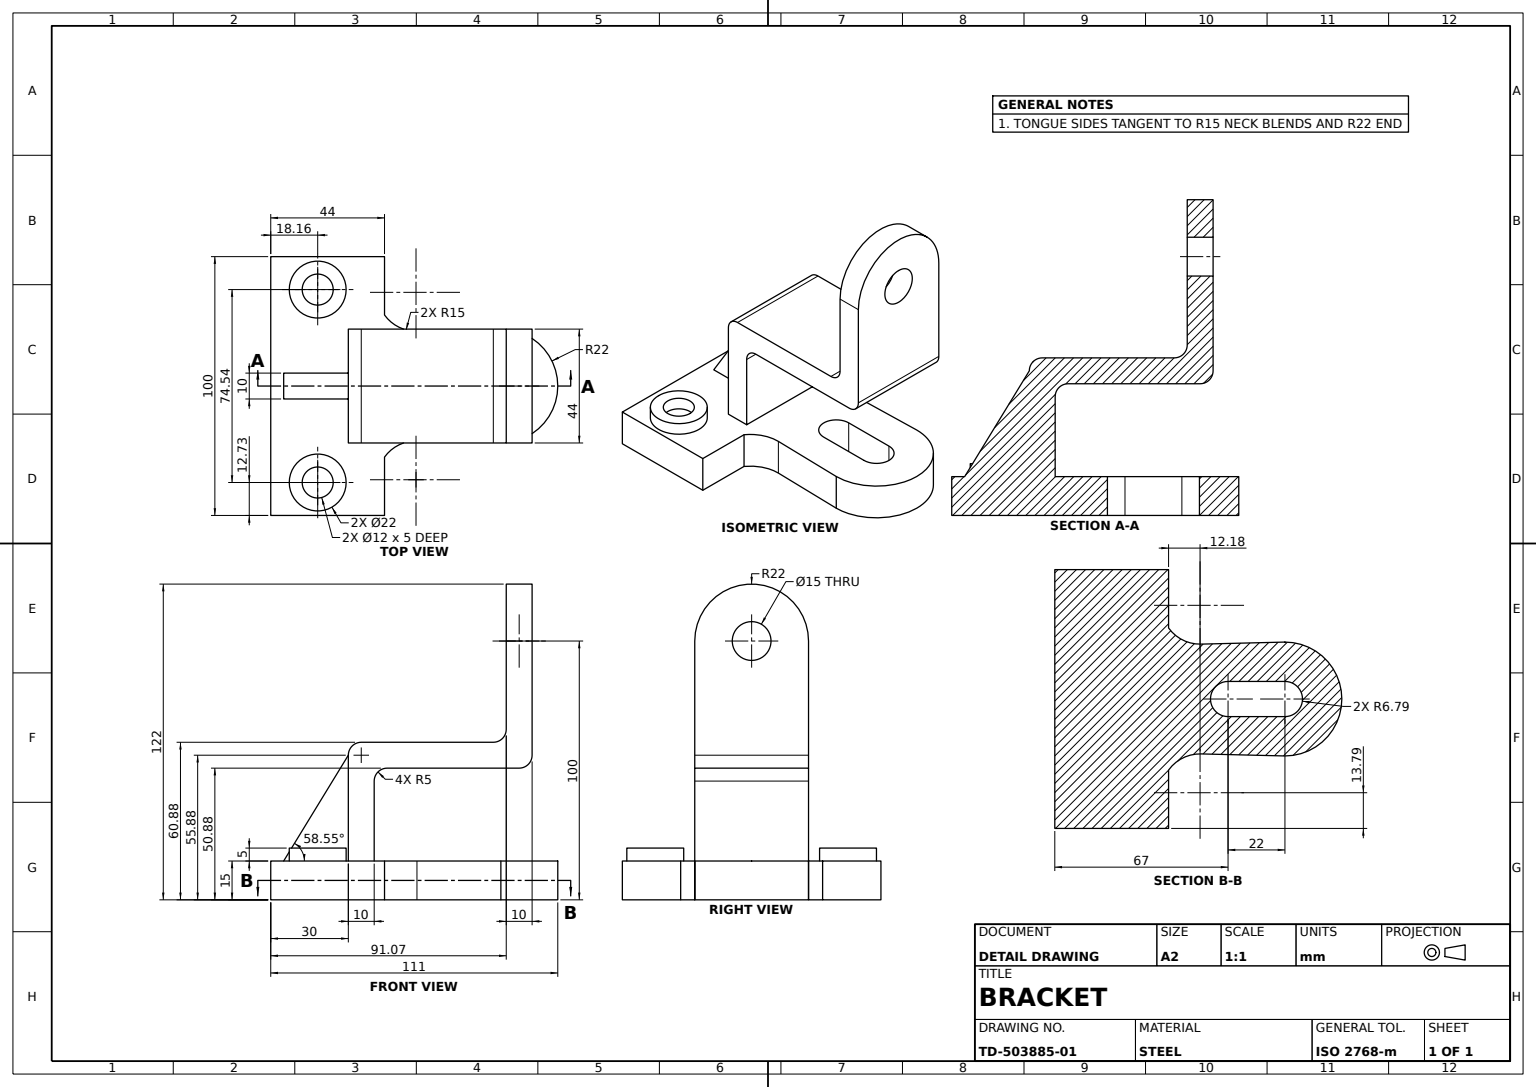
from build123d import *

# Parameters (mm, degrees)
BRACKET_PROFILE_SKETCH_W = 44
BRACKET_PROFILE_SKETCH_H = 15
BRACKET_BASE_BODY_DEPTH  = 50
UPRIGHT_WEB_DEPTH        = 22
LUG_BOSS_DEPTH           = 10
LUG_HOLE_CUT_DEPTH       = 44
WASHER_BOSS_SKETCH_R     = 11
WASHER_BOSS_SKETCH_R_2   = 6
WASHER_BOSS_22_DEPTH     = 5
WEB_PAD_DEPTH            = 5
SLOTTED_TAB_DEPTH        = 15


with BuildPart() as part:
    # Bracket Profile Sketch → Bracket Base Body (new, symmetric)
    with BuildSketch(Plane.XY):
        Rectangle(BRACKET_PROFILE_SKETCH_W, BRACKET_PROFILE_SKETCH_H)
    extrude(amount=BRACKET_BASE_BODY_DEPTH, both=True)

    # Sketch1_3 → Upright Web (add, symmetric)
    with BuildSketch(Plane.XY):
        with BuildLine():
            Line((8, 7.5), (18, 7.5))
            Line((18, 7.5), (18, 38.383152955))
            ThreePointArc((18, 38.383152955), (19.464466094, 41.91868686), (23, 43.383152955))
            Line((23, 43.383152955), (74.071731591, 43.383152955))
            ThreePointArc((74.071731591, 43.383152955), (77.607265497, 44.847619049), (79.071731591, 48.383152955))
            Line((79.071731591, 48.383152955), (79.071731591, 92.5))
            Line((79.071731591, 92.5), (69.071731591, 92.5))
            Line((69.071731591, 92.5), (69.071731591, 58.383152955))
            ThreePointArc((69.071731591, 58.383152955), (67.607265497, 54.847619049), (64.071731591, 53.383152955))
            Line((64.071731591, 53.383152955), (13, 53.383152955))
            ThreePointArc((13, 53.383152955), (9.464466094, 51.91868686), (8, 48.383152955))
            Line((8, 48.383152955), (8, 7.5))
        make_face()
    extrude(amount=UPRIGHT_WEB_DEPTH, both=True)

    # Lug Profile Sketch → Lug Boss (add)
    with BuildSketch(Plane.ZY.offset(-69.071731591)):
        with BuildLine():
            Line((7.5, 92.5), (22, 92.5))
            ThreePointArc((22, 92.5), (0, 114.5), (-22, 92.5))
            Line((-22, 92.5), (-7.5, 92.5))
            ThreePointArc((-7.5, 92.5), (0, 100), (7.5, 92.5))
        make_face()
    extrude(amount=-LUG_BOSS_DEPTH)

    # Sketch2_3 → Lug Hole Cut (cut)
    with BuildSketch(Plane.ZY.offset(-69.071731591)):
        with BuildLine():
            ThreePointArc((-7.5, 92.5), (0, 85), (7.5, 92.5))
            Line((7.5, 92.5), (-7.5, 92.5))
        make_face()
        with BuildLine():
            Line((-7.5, 92.5), (7.5, 92.5))
            ThreePointArc((7.5, 92.5), (0, 100), (-7.5, 92.5))
        make_face()
    extrude(amount=-LUG_HOLE_CUT_DEPTH, mode=Mode.SUBTRACT)

    # Washer Boss Sketch → Washer Boss _22 (add)
    # profile 1 of 2: a face of its own
    with BuildSketch(Plane(origin=(0, 7.5, 0), x_dir=(1, 0, 0), z_dir=(0, 1, 0))):
        with Locations((-3.843200035, 37.271330251)):
            Circle(WASHER_BOSS_SKETCH_R)
        with Locations(Location((-3.843200035, 37.271330251, 0), (0, 0, 180))):
            Circle(WASHER_BOSS_SKETCH_R_2, mode=Mode.SUBTRACT)
    # profile 2 of 2: a face of its own
    with BuildSketch(Plane(origin=(0, 7.5, 0), x_dir=(1, 0, 0), z_dir=(0, 1, 0))):
        with Locations((-3.843200035, -37.271330251)):
            Circle(WASHER_BOSS_SKETCH_R)
        with Locations((-3.843200035, -37.271330251)):
            Circle(WASHER_BOSS_SKETCH_R_2, mode=Mode.SUBTRACT)
    extrude(amount=WASHER_BOSS_22_DEPTH)

    # Web Pad Sketch → Web Pad (add, symmetric)
    with BuildSketch(Plane.XY):
        Polygon((8, 48.383152955), (-17, 7.5), (8, 7.5), align=None)
    extrude(amount=WEB_PAD_DEPTH, both=True)

    # Slotted Tab Sketch → Slotted Tab (add)
    with BuildSketch(Plane.XZ.offset(7.5)):
        with BuildLine():
            Line((66.991803694, 21.999998473), (34.541419601, 21.210572784))
            ThreePointArc((34.541419601, 21.210572784), (27.498169269, 22.774892965), (22, 27.446574412))
            Line((22, 27.446574412), (22, -27.446574412))
            ThreePointArc((22, -27.446574412), (27.498169269, -22.774892965), (34.541419601, -21.210572784))
            Line((34.541419601, -21.210572784), (66.991803694, -21.999998473))
            ThreePointArc((66.991803694, -21.999998473), (89, 0), (66.991803694, 21.999998473))
        make_face()
        with BuildLine():
            ThreePointArc((67, 6.793312715), (73.793312715, 0), (67, -6.793312715))
            Line((67, -6.793312715), (45, -6.793312715))
            ThreePointArc((45, -6.793312715), (38.206687285, 0), (45, 6.793312715))
            Line((45, 6.793312715), (67, 6.793312715))
        make_face(mode=Mode.SUBTRACT)
    extrude(amount=-SLOTTED_TAB_DEPTH)


solid = part.part
